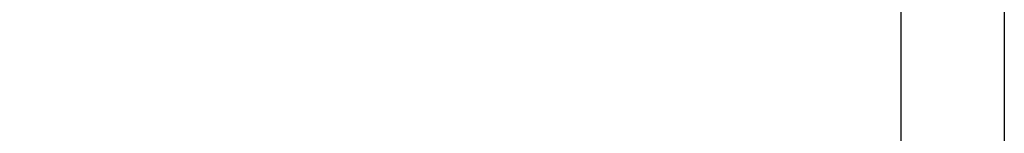
# Model space of a CAD drawing. Units: inches. Extents: x 2091 to 2899, y 967 to 2217.
# Tile 33 of 256: x 2390 to 2459, y 1081 to 1089. Entities that reach past the tile are written whole.
import ezdxf

# ---------------------------------------------------------------- set-up
doc = ezdxf.new("R2010")
doc.units = ezdxf.units.IN
doc.layers.add('A-ANNO-DIMS', color=2, linetype='Continuous', lineweight=18)
doc.styles.get("Standard").update_dxf_attribs({"font": 'arial.ttf'})
doc.dimstyles.new('ISO-25', dxfattribs={"dimtxt": 4, "dimasz": 4, "dimexe": 1.25, "dimexo": 0.625, "dimtad": 1, "dimdec": 0, "dimlunit": 3, "dimtxsty": 'Standard', "dimcen": 2.5, "dimadec": 0, "dimazin": 0, "dimtfac": 1, "dimtdec": 0, "dimtmove": 0, "dimatfit": 3, "dimfxl": 1, "dimarcsym": 0})

# ---------------------------------------------------------------- blocks, each defined once
blk = doc.blocks.new('*D68')
at = {"layer": 'A-ANNO-DIMS', "color": 0, "lineweight": -2, "transparency": 16777216}
for p, q in [((2317.144, 1535.794), (2317.144, 969.464)), ((2459.384, 1535.794), (2459.384, 969.464)), ((2321.144, 970.714), (2455.384, 970.714))]:
    blk.add_line(p, q, dxfattribs=at)
at = {"layer": 'A-ANNO-DIMS', "color": 0, "transparency": 16777216}
for points in [[(2321.144, 971.381), (2321.144, 970.048), (2317.144, 970.714)], [(2455.384, 971.381), (2455.384, 970.048), (2459.384, 970.714)]]:
    blk.add_solid(points, dxfattribs=at)
at = {"layer": 'Defpoints', "color": 0, "transparency": 16777216}
for p in [(2317.144, 1536.419), (2459.384, 1536.419), (2459.384, 970.714)]:
    blk.add_point(p, dxfattribs=at)
at = {"layer": 'A-ANNO-DIMS', "color": 0, "transparency": 16777216, "insert": (2388.264, 973.382), "char_height": 4, "attachment_point": 5}
blk.add_mtext('11\'-10"', dxfattribs=at)
blk = doc.blocks.new('*D71')
at = {"layer": 'A-ANNO-DIMS', "color": 0, "lineweight": -2, "transparency": 16777216}
for p, q in [((2212.144, 1351.294), (2212.144, 969.464)), ((2452.144, 1351.294), (2452.144, 969.464)), ((2216.144, 970.714), (2448.144, 970.714))]:
    blk.add_line(p, q, dxfattribs=at)
at = {"layer": 'A-ANNO-DIMS', "color": 0, "transparency": 16777216}
for points in [[(2216.144, 971.381), (2216.144, 970.048), (2212.144, 970.714)], [(2448.144, 971.381), (2448.144, 970.048), (2452.144, 970.714)]]:
    blk.add_solid(points, dxfattribs=at)
at = {"layer": 'Defpoints', "color": 0, "transparency": 16777216}
for p in [(2212.144, 1351.919), (2452.144, 1351.919), (2452.144, 970.714)]:
    blk.add_point(p, dxfattribs=at)
at = {"layer": 'A-ANNO-DIMS', "color": 0, "transparency": 16777216, "insert": (2332.144, 973.382), "char_height": 4, "attachment_point": 5}
blk.add_mtext('20\'-0"', dxfattribs=at)

msp = doc.modelspace()

# ---------------------------------------------------------------- dimensions: what is measured, and where the dimension line sits
at = {"layer": 'A-ANNO-DIMS'}
for base, p1, p2, picture, middle in [((2459.384, 970.714), (2317.144, 1536.419), (2459.384, 1536.419), '*D68', (2388.264, 973.382)), ((2452.144, 970.714), (2212.144, 1351.919), (2452.144, 1351.919), '*D71', (2332.144, 973.382))]:
    dim = msp.add_linear_dim(base=base, p1=p1, p2=p2, dimstyle='ISO-25', override={"dimdec": 1, "dimlfac": 1, "dimrnd": 0, "dimzin": 1, "dimdsep": 46, "dimlunit": 4, "dimfrac": 2}, dxfattribs=at)
    dim.commit()
    dim.dimension.update_dxf_attribs({"geometry": picture, "text_midpoint": middle})

doc.saveas('drawing.dxf')
